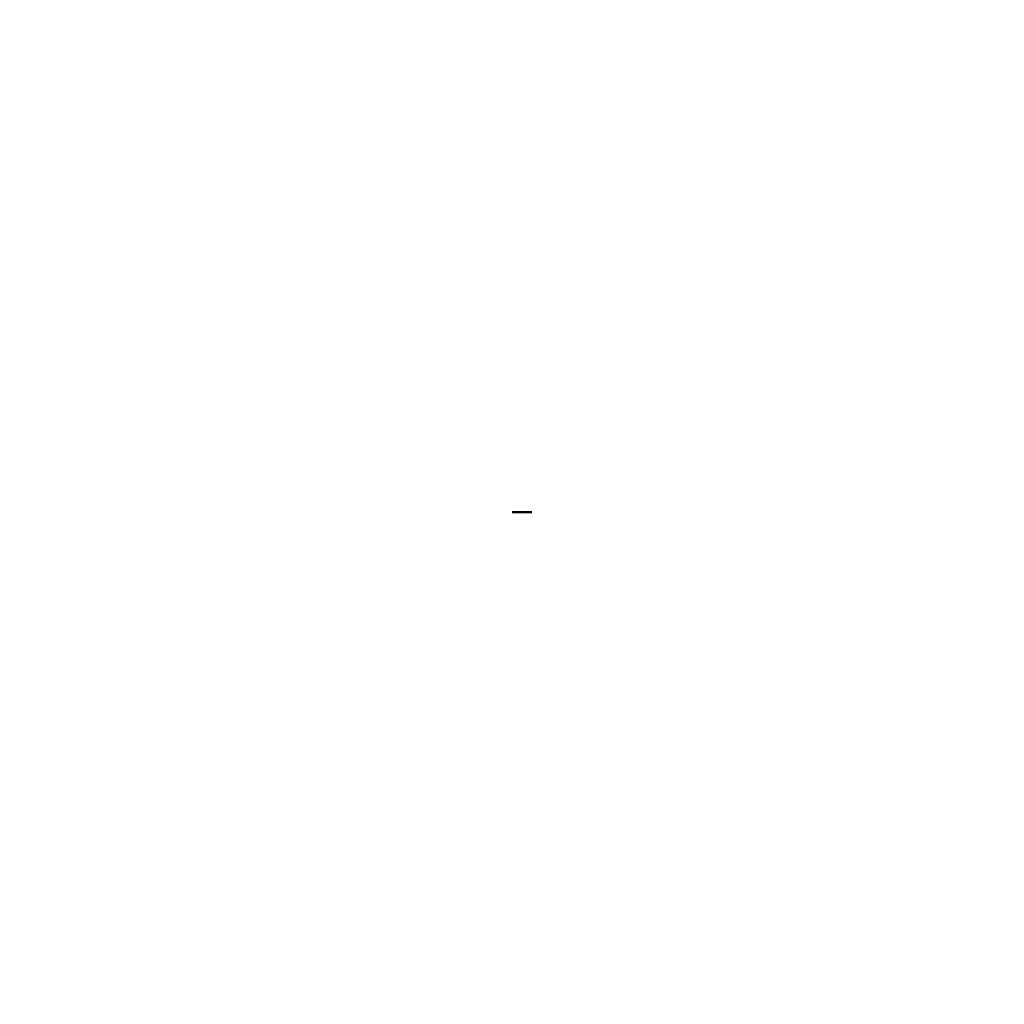
# Model space of a CAD drawing. Units: millimetres. Extents: x -25 to 763, y -62 to 306.
# Tile 1 of 7: x -25 to 25, y -25 to 25. Entities that reach past the tile are written whole.
import ezdxf

# ---------------------------------------------------------------- set-up
doc = ezdxf.new("R2010")
doc.units = ezdxf.units.MM
doc.header["$LTSCALE"] = 0.5
doc.layers.add('M-OUTL', color=7, linetype='Continuous', lineweight=50)

msp = doc.modelspace()

# ---------------------------------------------------------------- linework, layer by layer
at = {"layer": 'M-OUTL', "ltscale": 0.5}
for radius in [25, 15, 12.623]:
    msp.add_arc((0, 0), radius, 0, 0, dxfattribs=at)
at = {"layer": 'M-OUTL'}
for radius in [6, 5, 2, 2]:
    msp.add_arc((0, 0), radius, 0, 0, dxfattribs=at)
msp.add_open_spline([(0, 0), (0.333, 0), (0.667, 0), (1, 0)], degree=3, dxfattribs=at)

doc.saveas('drawing.dxf')
